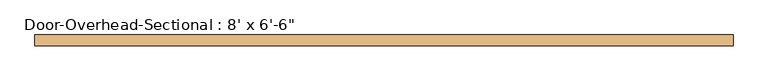
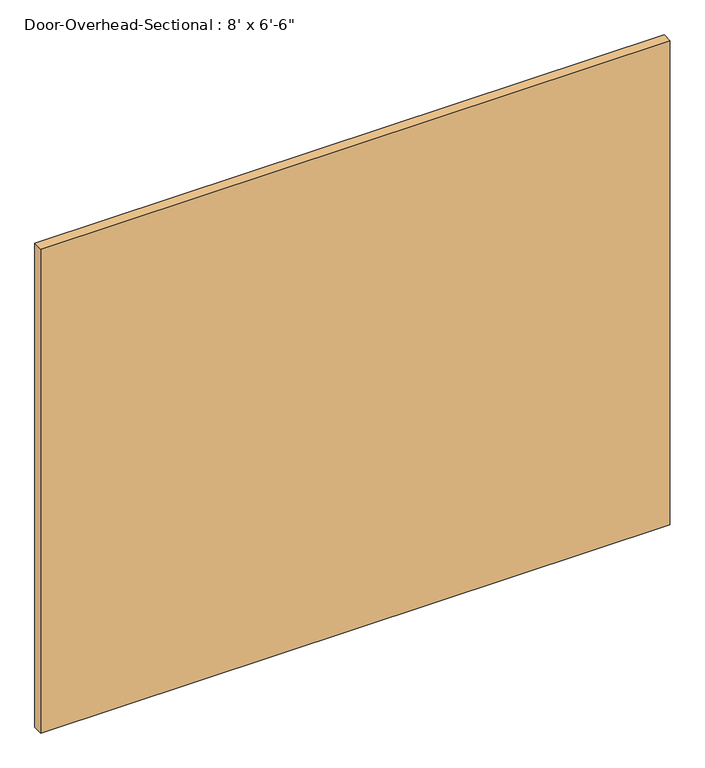
"""IFC4 building model written with IfcOpenShell, lengths in millimetres: door geometry."""

from ifc_helpers import new_model, si_unit, origin, origin_with_axes, place, context, project, spatial, polyline, outline, extrude, source, transform, mapped, element, save


def door_8b017a1a(model_context):
    return source(origin(), model_context, "Body", "SweptSolid", [
        extrude(outline(polyline([(1219.2, 50.8), (-1219.2, 50.8), (-1219.2, 88.9), (1219.2, 88.9), (1219.2, 50.8)])), origin_with_axes(), (0.0, 0.0, 1.0), 1981.2),
    ])


if __name__ == "__main__":
    model = new_model("IFC4")
    model_context = context("Model", 3, world=origin())
    ifc_project = project(units=[si_unit("LENGTHUNIT", "METRE", prefix="MILLI")], contexts=[model_context])
    site = spatial("IfcSite", under=ifc_project)
    building = spatial("IfcBuilding", under=site)
    placement = place(None, origin())
    door_shape = door_8b017a1a(model_context)
    element("IfcDoor", 1, ObjectType="Door-Overhead-Sectional : 8' x 6'-6\"", at=placement, inside=building, context=model_context, shape_type="MappedRepresentation", body=[
        mapped(door_shape, transform((0.0, 0.0, 0.0), x_axis=(1.0, 0.0, 0.0), y_axis=(0.0, 1.0, 0.0), z_axis=(0.0, 0.0, 1.0))),
    ])
    save(model, "model.ifc")

# Revit data of these elements
# Type "Door-Overhead-Sectional : 8' x 6'-6\""
#   Type Mark = "9"
#   Construction Type Id = "MDOOR"
#   Assembly Code = "B2030400"
#   Analytic Construction = "Metal"
#   Rough Width [instance default] = 8' - 0"
#   Rough Height [instance default] = 6' - 6"
#   Heat Transfer Coefficient (U) = 0.651978 BTU/(h·ft²·°F)
#   Height [instance default] = 6' - 6"
#   Thickness = 0' - 1 1/2"
#   Width [instance default] = 8' - 0"
#   Define Thermal Properties by = 1
#   Function = 1
#   Panel Material = Steel, Paint Finish, Ivory, Matte
#   Visual Light Transmittance = 0
#   Solar Heat Gain Coefficient = 0
#   Wall Closure = (empty or 0)
# Element 1 (IfcDoor, "Door-Overhead-Sectional : 8' x 6'-6\"")
#   Materials on its faces: "Steel, Paint Finish, Ivory, Matte"
# Materials
#   "Steel, Paint Finish, Ivory, Matte": class "Metal", colour RGB 247 247 239, transparency 0, Description = "Steel, paint finish, ivory, matte", Cost = 0
